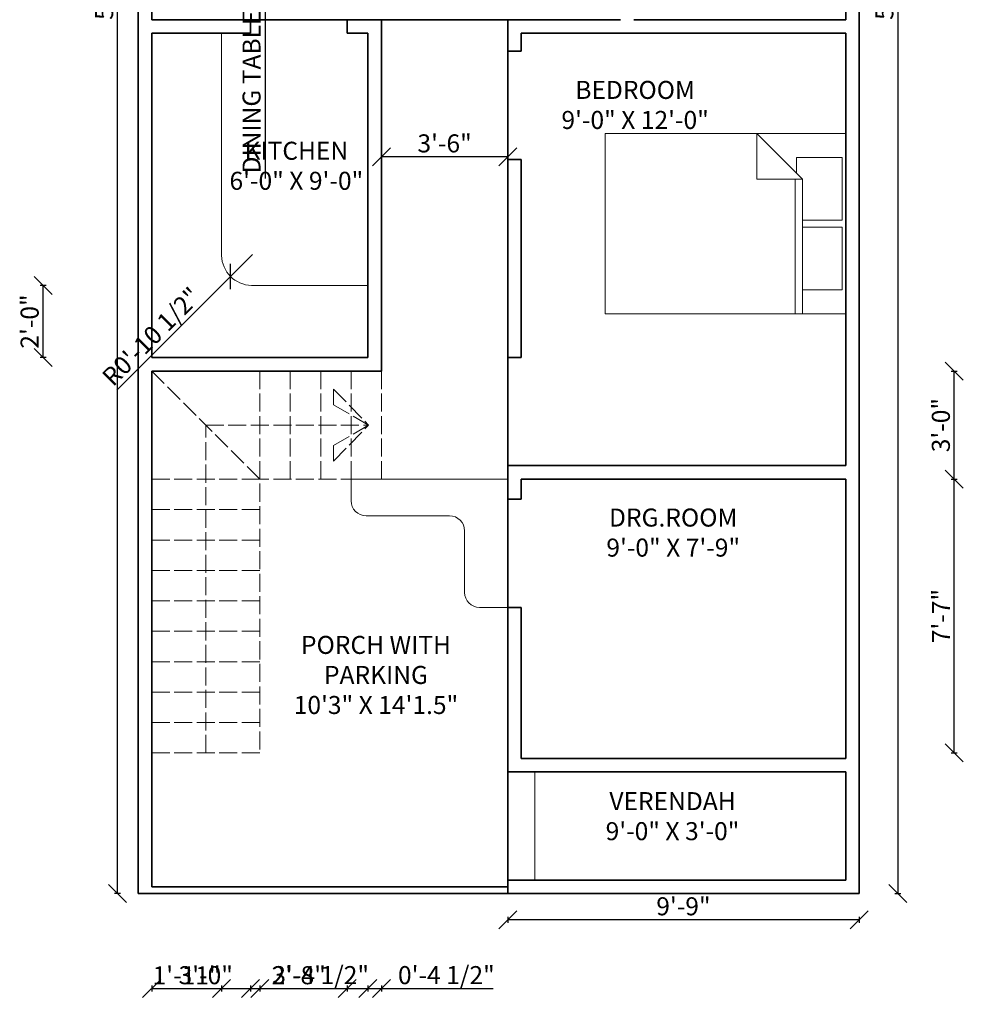
# Model space of a CAD drawing. Units: inches. Extents: x 2598 to 3019, y 330 to 985.
# Tile 1 of 2: x 2650 to 2964, y 330 to 657. Entities that reach past the tile are written whole.
import ezdxf

# ---------------------------------------------------------------- set-up
doc = ezdxf.new("R2010")
doc.units = ezdxf.units.IN
doc.linetypes.add('ACAD_ISO02W100', pattern=[15, 12, -3])
for name, color, linetype, lineweight in [('A-ANNO-DIMS', 2, 'Continuous', 13), ('A-AREA-IDEN', 114, 'Continuous', 18), ('A-FLOR', 7, 'Continuous', 18), ('A-FLOR-CASE', 8, 'Continuous', 18), ('A-FLOR-STRS', 212, 'ACAD_ISO02W100', 18), ('A-FURN', 8, 'Continuous', 18), ('A-WALL', 7, 'Continuous', 35)]:
    doc.layers.add(name, color=color, linetype=linetype, lineweight=lineweight)
doc.styles.get("Standard").update_dxf_attribs({"font": 'arial.ttf'})
doc.dimstyles.new('ISO-25', dxfattribs={"dimtxt": 6, "dimasz": 6, "dimexe": 1, "dimexo": 3, "dimtad": 1, "dimlunit": 3, "dimtxsty": 'Standard', "dimblk": 'OBLIQUE', "dimcen": 2.5, "dimclrt": 6, "dimadec": 0, "dimazin": 0, "dimtfac": 1, "dimtmove": 0, "dimatfit": 3, "dimfxl": 1, "dimfxlon": 1, "dimarcsym": 0})

# ---------------------------------------------------------------- blocks, each defined once
blk = doc.blocks.new('_Oblique')
at = {"color": 0, "linetype": 'ByBlock', "lineweight": -2}
blk.add_line((-0.5, -0.5), (0.5, 0.5), dxfattribs=at)
blk = doc.blocks.new('*D4')
at = {"layer": 'A-ANNO-DIMS', "color": 0, "lineweight": -2, "transparency": 16777216}
for p, q in [((2940.88, 970.94), (2942.88, 970.94)), ((2941.88, 970.94), (2941.88, 366.44)), ((2940.88, 366.44), (2942.88, 366.44))]:
    blk.add_line(p, q, dxfattribs=at)
at = {"layer": 'Defpoints', "color": 0, "transparency": 16777216}
for p in [(2929.06, 970.94), (2929.06, 366.44), (2941.88, 366.44)]:
    blk.add_point(p, dxfattribs=at)
at = {"layer": 'A-ANNO-DIMS', "color": 0, "lineweight": -2, "transparency": 16777216, "xscale": 6, "yscale": 6, "zscale": 6}
for p, rotation in [((2941.88, 970.94), 90), ((2941.88, 366.44), 270)]:
    blk.add_blockref('_Oblique', p, dxfattribs=dict(at, rotation=rotation))
at = {"layer": 'A-ANNO-DIMS', "color": 0, "transparency": 16777216, "insert": (2938.2, 668.69), "char_height": 6, "attachment_point": 5, "rotation": 90}
blk.add_mtext('50\'-0"', dxfattribs=at)
blk = doc.blocks.new('*D5')
at = {"layer": 'A-ANNO-DIMS', "color": 0, "lineweight": -2, "transparency": 16777216}
for p, q in [((2770.06, 611.78), (2770.06, 612.78)), ((2812.06, 611.78), (2770.06, 611.78)), ((2812.06, 611.78), (2812.06, 612.78))]:
    blk.add_line(p, q, dxfattribs=at)
at = {"layer": 'Defpoints', "color": 0, "transparency": 16777216}
for p in [(2770.06, 611.78), (2770.06, 610.94), (2812.06, 610.94)]:
    blk.add_point(p, dxfattribs=at)
at = {"layer": 'A-ANNO-DIMS', "color": 0, "lineweight": -2, "transparency": 16777216, "xscale": 6, "yscale": 6, "zscale": 6, "rotation": 180}
blk.add_blockref('_Oblique', (2770.06, 611.78), dxfattribs=at)
at = {"layer": 'A-ANNO-DIMS', "color": 0, "lineweight": -2, "transparency": 16777216, "xscale": 6, "yscale": 6, "zscale": 6}
blk.add_blockref('_Oblique', (2812.06, 611.78), dxfattribs=at)
at = {"layer": 'A-ANNO-DIMS', "color": 0, "transparency": 16777216, "insert": (2791.06, 615.48), "char_height": 6, "attachment_point": 5}
blk.add_mtext('3\'-6"', dxfattribs=at)
blk = doc.blocks.new('*D6')
at = {"layer": 'A-ANNO-DIMS', "color": 0, "lineweight": -2, "transparency": 16777216}
for p, q in [((2812.06, 358.75), (2812.06, 356.75)), ((2929.06, 357.75), (2812.06, 357.75)), ((2929.06, 358.75), (2929.06, 356.75))]:
    blk.add_line(p, q, dxfattribs=at)
at = {"layer": 'Defpoints', "color": 0, "transparency": 16777216}
for p in [(2812.06, 366.44), (2929.06, 366.44), (2812.06, 357.75)]:
    blk.add_point(p, dxfattribs=at)
at = {"layer": 'A-ANNO-DIMS', "color": 0, "lineweight": -2, "transparency": 16777216, "xscale": 6, "yscale": 6, "zscale": 6, "rotation": 180}
blk.add_blockref('_Oblique', (2812.06, 357.75), dxfattribs=at)
at = {"layer": 'A-ANNO-DIMS', "color": 0, "lineweight": -2, "transparency": 16777216, "xscale": 6, "yscale": 6, "zscale": 6}
blk.add_blockref('_Oblique', (2929.06, 357.75), dxfattribs=at)
at = {"layer": 'A-ANNO-DIMS', "color": 0, "transparency": 16777216, "insert": (2870.56, 361.44), "char_height": 6, "attachment_point": 5}
blk.add_mtext('9\'-9"', dxfattribs=at)
blk = doc.blocks.new('Bed - Queen')
for p, q in [((0, -80.00003), (0, 0)), ((0, 0), (59.99999, 0)), ((59.99999, 0), (59.99999, -80.00003)), ((7.99999, -1.2), (28.79998, -1.2)), ((7.99999, -14.4), (7.99999, -1.2)), ((28.79998, -1.2), (28.79998, -14.4)), ((31.19999, -1.2), (51.99999, -1.2)), ((31.19999, -14.4), (31.19999, -1.2)), ((51.99999, -1.2), (51.99999, -16.4)), ((0, -14.4), (44.8, -14.4)), ((59.99999, -29.6), (44.8, -14.4)), ((44.8, -14.4), (44.8, -29.6)), ((44.8, -16.8), (0, -16.8)), ((51.99999, -16.4), (46.79936, -16.4)), ((44.8, -29.6), (59.99999, -29.6)), ((59.99999, -80.00003), (0, -80.00003))]:
    blk.add_line(p, q)
blk = doc.blocks.new('*D15')
at = {"layer": 'A-ANNO-DIMS', "color": 0, "lineweight": -2, "transparency": 16777216}
for p, q in [((2683.19, 970.94), (2681.19, 970.94)), ((2682.19, 366.44), (2682.19, 970.94)), ((2683.19, 366.44), (2681.19, 366.44))]:
    blk.add_line(p, q, dxfattribs=at)
at = {"layer": 'Defpoints', "color": 0, "transparency": 16777216}
for p in [(2682.19, 970.94), (2689.06, 970.94), (2689.06, 366.44)]:
    blk.add_point(p, dxfattribs=at)
at = {"layer": 'A-ANNO-DIMS', "color": 0, "lineweight": -2, "transparency": 16777216, "xscale": 6, "yscale": 6, "zscale": 6}
for p, rotation in [((2682.19, 970.94), 90), ((2682.19, 366.44), 270)]:
    blk.add_blockref('_Oblique', p, dxfattribs=dict(at, rotation=rotation))
at = {"layer": 'A-ANNO-DIMS', "color": 0, "transparency": 16777216, "insert": (2678.5, 668.69), "char_height": 6, "attachment_point": 5, "rotation": 90}
blk.add_mtext('50\'-0"', dxfattribs=at)
blk = doc.blocks.new('*D25')
at = {"layer": 'A-ANNO-DIMS', "color": 0, "lineweight": -2, "transparency": 16777216}
for p, q in [((2732.31, 748.04), (2730.31, 748.04)), ((2731.31, 748.04), (2731.31, 688.04)), ((2732.31, 688.04), (2730.31, 688.04)), ((2731.31, 688.04), (2731.31, 604.59))]:
    blk.add_line(p, q, dxfattribs=at)
at = {"layer": 'Defpoints', "color": 0, "transparency": 16777216}
for p in [(2740.31, 748.04), (2731.31, 688.04), (2740.31, 688.04)]:
    blk.add_point(p, dxfattribs=at)
at = {"layer": 'A-ANNO-DIMS', "color": 0, "lineweight": -2, "transparency": 16777216, "xscale": 6, "yscale": 6, "zscale": 6}
for p, rotation in [((2731.31, 748.04), 90), ((2731.31, 688.04), 270)]:
    blk.add_blockref('_Oblique', p, dxfattribs=dict(at, rotation=rotation))
at = {"layer": 'A-ANNO-DIMS', "color": 6, "transparency": 16777216, "insert": (2727.58, 643.32), "char_height": 6, "attachment_point": 5, "rotation": 90}
blk.add_mtext('DINING TABLE 5\'-0"', dxfattribs=at)
blk = doc.blocks.new('*D27')
at = {"layer": 'A-ANNO-DIMS', "color": 0, "lineweight": -2, "transparency": 16777216}
for p, q in [((2693.56, 335.79), (2693.56, 333.79)), ((2693.56, 334.79), (2729.56, 334.79)), ((2729.56, 335.79), (2729.56, 333.79))]:
    blk.add_line(p, q, dxfattribs=at)
at = {"layer": 'Defpoints', "color": 0, "transparency": 16777216}
for p in [(2693.56, 413.27), (2729.56, 413.27), (2729.56, 334.79)]:
    blk.add_point(p, dxfattribs=at)
at = {"layer": 'A-ANNO-DIMS', "color": 0, "lineweight": -2, "transparency": 16777216, "xscale": 6, "yscale": 6, "zscale": 6, "rotation": 180}
blk.add_blockref('_Oblique', (2693.56, 334.79), dxfattribs=at)
at = {"layer": 'A-ANNO-DIMS', "color": 0, "lineweight": -2, "transparency": 16777216, "xscale": 6, "yscale": 6, "zscale": 6}
blk.add_blockref('_Oblique', (2729.56, 334.79), dxfattribs=at)
at = {"layer": 'A-ANNO-DIMS', "color": 6, "transparency": 16777216, "insert": (2711.56, 338.49), "char_height": 6, "attachment_point": 5}
blk.add_mtext('3\'-0"', dxfattribs=at)
blk = doc.blocks.new('*D28')
at = {"layer": 'A-ANNO-DIMS', "color": 0, "lineweight": -2, "transparency": 16777216}
for p, q in [((2959.711602, 504.44461), (2961.711602, 504.44461)), ((2960.711602, 413.27461), (2960.711602, 504.44461)), ((2959.711602, 413.27461), (2961.711602, 413.27461))]:
    blk.add_line(p, q, dxfattribs=at)
at = {"layer": 'Defpoints', "color": 0, "transparency": 16777216}
for p in [(2729.561602, 504.44461), (2960.711602, 504.44461), (2729.561602, 413.27461)]:
    blk.add_point(p, dxfattribs=at)
at = {"layer": 'A-ANNO-DIMS', "color": 0, "lineweight": -2, "transparency": 16777216, "xscale": 6, "yscale": 6, "zscale": 6}
for p, rotation in [((2960.711602, 504.44461), 90), ((2960.711602, 413.27461), 270)]:
    blk.add_blockref('_Oblique', p, dxfattribs=dict(at, rotation=rotation))
at = {"layer": 'A-ANNO-DIMS', "color": 6, "transparency": 16777216, "insert": (2957.086602, 458.85961), "char_height": 6, "attachment_point": 5, "rotation": 90}
blk.add_mtext('7\'-7"', dxfattribs=at)
blk = doc.blocks.new('*D29')
at = {"layer": 'A-ANNO-DIMS', "color": 0, "lineweight": -2, "transparency": 16777216}
for p, q in [((2959.71, 540.44), (2961.71, 540.44)), ((2960.71, 504.44), (2960.71, 540.44)), ((2959.71, 504.44), (2961.71, 504.44))]:
    blk.add_line(p, q, dxfattribs=at)
at = {"layer": 'Defpoints', "color": 0, "transparency": 16777216}
for p in [(2770.06, 540.44), (2960.71, 540.44), (2770.06, 504.44)]:
    blk.add_point(p, dxfattribs=at)
at = {"layer": 'A-ANNO-DIMS', "color": 0, "lineweight": -2, "transparency": 16777216, "xscale": 6, "yscale": 6, "zscale": 6}
for p, rotation in [((2960.71, 540.44), 90), ((2960.71, 504.44), 270)]:
    blk.add_blockref('_Oblique', p, dxfattribs=dict(at, rotation=rotation))
at = {"layer": 'A-ANNO-DIMS', "color": 6, "transparency": 16777216, "insert": (2957.02, 522.44), "char_height": 6, "attachment_point": 5, "rotation": 90}
blk.add_mtext('3\'-0"', dxfattribs=at)
blk = doc.blocks.new('*D30')
at = {"layer": 'A-ANNO-DIMS', "color": 0, "lineweight": -2, "transparency": 16777216}
for p, q in [((2729.56, 335.79), (2729.56, 333.79)), ((2729.56, 334.79), (2770.06, 334.79)), ((2770.06, 335.79), (2770.06, 333.79))]:
    blk.add_line(p, q, dxfattribs=at)
at = {"layer": 'Defpoints', "color": 0, "transparency": 16777216}
for p in [(2729.56, 504.44), (2770.06, 504.44), (2770.06, 334.79)]:
    blk.add_point(p, dxfattribs=at)
at = {"layer": 'A-ANNO-DIMS', "color": 0, "lineweight": -2, "transparency": 16777216, "xscale": 6, "yscale": 6, "zscale": 6, "rotation": 180}
blk.add_blockref('_Oblique', (2729.56, 334.79), dxfattribs=at)
at = {"layer": 'A-ANNO-DIMS', "color": 0, "lineweight": -2, "transparency": 16777216, "xscale": 6, "yscale": 6, "zscale": 6}
blk.add_blockref('_Oblique', (2770.06, 334.79), dxfattribs=at)
at = {"layer": 'A-ANNO-DIMS', "color": 6, "transparency": 16777216, "insert": (2749.81, 338.52), "char_height": 6, "attachment_point": 5}
blk.add_mtext('3\'-4 1/2"', dxfattribs=at)
blk = doc.blocks.new('*D31')
at = {"layer": 'A-ANNO-DIMS', "color": 0, "lineweight": -2, "transparency": 16777216}
for p, q in [((2693.56, 335.79), (2693.56, 333.79)), ((2693.56, 334.79), (2716.8, 334.79)), ((2716.8, 335.79), (2716.8, 333.79))]:
    blk.add_line(p, q, dxfattribs=at)
at = {"layer": 'Defpoints', "color": 0, "transparency": 16777216}
for p in [(2693.56, 652.94), (2716.8, 652.94), (2716.8, 334.79)]:
    blk.add_point(p, dxfattribs=at)
at = {"layer": 'A-ANNO-DIMS', "color": 0, "lineweight": -2, "transparency": 16777216, "xscale": 6, "yscale": 6, "zscale": 6, "rotation": 180}
blk.add_blockref('_Oblique', (2693.56, 334.79), dxfattribs=at)
at = {"layer": 'A-ANNO-DIMS', "color": 0, "lineweight": -2, "transparency": 16777216, "xscale": 6, "yscale": 6, "zscale": 6}
blk.add_blockref('_Oblique', (2716.8, 334.79), dxfattribs=at)
at = {"layer": 'A-ANNO-DIMS', "color": 6, "transparency": 16777216, "insert": (2705.18, 338.43), "char_height": 6, "attachment_point": 5}
blk.add_mtext('1\'-11"', dxfattribs=at)
blk = doc.blocks.new('*D32')
at = {"layer": 'A-ANNO-DIMS', "color": 0, "lineweight": -2, "transparency": 16777216}
for p, q in [((2658.41, 568.94), (2656.41, 568.94)), ((2657.41, 544.94), (2657.41, 568.94)), ((2658.41, 544.94), (2656.41, 544.94))]:
    blk.add_line(p, q, dxfattribs=at)
at = {"layer": 'Defpoints', "color": 0, "transparency": 16777216}
for p in [(2657.41, 568.94), (2765.56, 568.94), (2765.56, 544.94)]:
    blk.add_point(p, dxfattribs=at)
at = {"layer": 'A-ANNO-DIMS', "color": 0, "lineweight": -2, "transparency": 16777216, "xscale": 6, "yscale": 6, "zscale": 6}
for p, rotation in [((2657.41, 568.94), 90), ((2657.41, 544.94), 270)]:
    blk.add_blockref('_Oblique', p, dxfattribs=dict(at, rotation=rotation))
at = {"layer": 'A-ANNO-DIMS', "color": 6, "transparency": 16777216, "insert": (2653.72, 556.94), "char_height": 6, "attachment_point": 5, "rotation": 90}
blk.add_mtext('2\'-0"', dxfattribs=at)
blk = doc.blocks.new('*D33')
at = {"layer": 'A-ANNO-DIMS', "color": 0, "lineweight": -2, "transparency": 16777216}
for p, q in [((2726.42, 335.79), (2726.42, 333.79)), ((2726.42, 334.79), (2758.6, 334.79)), ((2758.6, 335.79), (2758.6, 333.79))]:
    blk.add_line(p, q, dxfattribs=at)
at = {"layer": 'Defpoints', "color": 0, "transparency": 16777216}
for p in [(2726.42, 652.94), (2758.6, 652.94), (2758.6, 334.79)]:
    blk.add_point(p, dxfattribs=at)
at = {"layer": 'A-ANNO-DIMS', "color": 0, "lineweight": -2, "transparency": 16777216, "xscale": 6, "yscale": 6, "zscale": 6, "rotation": 180}
blk.add_blockref('_Oblique', (2726.42, 334.79), dxfattribs=at)
at = {"layer": 'A-ANNO-DIMS', "color": 0, "lineweight": -2, "transparency": 16777216, "xscale": 6, "yscale": 6, "zscale": 6}
blk.add_blockref('_Oblique', (2758.6, 334.79), dxfattribs=at)
at = {"layer": 'A-ANNO-DIMS', "color": 6, "transparency": 16777216, "insert": (2742.51, 338.48), "char_height": 6, "attachment_point": 5}
blk.add_mtext('2\'-8"', dxfattribs=at)
blk = doc.blocks.new('*D34')
at = {"layer": 'A-ANNO-DIMS', "color": 0, "lineweight": -2, "transparency": 16777216}
for p, q in [((2765.56, 335.79), (2765.56, 333.79)), ((2765.56, 334.79), (2770.06, 334.79)), ((2770.06, 335.79), (2770.06, 333.79)), ((2770.06, 334.79), (2807.24, 334.79))]:
    blk.add_line(p, q, dxfattribs=at)
at = {"layer": 'Defpoints', "color": 0, "transparency": 16777216}
for p in [(2765.56, 544.94), (2770.06, 540.44), (2770.06, 334.79)]:
    blk.add_point(p, dxfattribs=at)
at = {"layer": 'A-ANNO-DIMS', "color": 0, "lineweight": -2, "transparency": 16777216, "xscale": 6, "yscale": 6, "zscale": 6, "rotation": 180}
blk.add_blockref('_Oblique', (2765.56, 334.79), dxfattribs=at)
at = {"layer": 'A-ANNO-DIMS', "color": 0, "lineweight": -2, "transparency": 16777216, "xscale": 6, "yscale": 6, "zscale": 6}
blk.add_blockref('_Oblique', (2770.06, 334.79), dxfattribs=at)
at = {"layer": 'A-ANNO-DIMS', "color": 6, "transparency": 16777216, "insert": (2791.65, 338.52), "char_height": 6, "attachment_point": 5}
blk.add_mtext('0\'-4 1/2"', dxfattribs=at)
blk = doc.blocks.new('*D39')
at = {"layer": 'A-ANNO-DIMS', "color": 0, "lineweight": -2, "transparency": 16777216}
for p in [(2727.08, 579.22), (2681.92, 534.06)]:
    blk.add_line(p, (2719.81, 571.95), dxfattribs=at)
at = {"layer": 'Defpoints', "color": 0, "transparency": 16777216}
for p in [(2727.08, 579.22), (2719.81, 571.95)]:
    blk.add_point(p, dxfattribs=at)
at = {"layer": 'A-ANNO-DIMS', "color": 0, "lineweight": -2, "transparency": 16777216, "xscale": 6, "yscale": 6, "zscale": 6, "rotation": 44.99835699208987}
blk.add_blockref('_Oblique', (2719.81, 571.95), dxfattribs=at)
at = {"layer": 'A-ANNO-DIMS', "color": 6, "transparency": 16777216, "insert": (2693.99, 551.4), "char_height": 6, "attachment_point": 5, "rotation": 44.9984}
blk.add_mtext('R0\'-10 1/2"', dxfattribs=at)

msp = doc.modelspace()

# ---------------------------------------------------------------- linework, layer by layer
at = {"layer": 'A-FLOR'}
for p, q in [((2759.937, 504.445), (2812.062, 504.445)), ((2759.937, 504.445), (2759.937, 497.246)), ((2764.937, 492.246), (2792.719, 492.246)), ((2797.719, 487.246), (2797.719, 466.758)), ((2802.719, 461.758), (2812.062, 461.758)), ((2821.062, 370.945), (2821.062, 406.945))]:
    msp.add_line(p, q, dxfattribs=at)
for centre, start, end in [((2764.937, 497.246), 180, 270), ((2792.719, 487.246), 0, 90), ((2802.719, 466.758), 180, 270)]:
    msp.add_arc(centre, 5, start, end, dxfattribs=at)
at = {"layer": 'A-FLOR-CASE'}
for p, q in [((2716.803, 652.945), (2716.803, 578.945)), ((2726.803, 568.945), (2765.562, 568.945))]:
    msp.add_line(p, q, dxfattribs=at)
msp.add_arc((2727.082, 579.223), 10.283, 181.55394, 268.44606, dxfattribs=at)
at = {"layer": 'A-FLOR-STRS', "ltscale": 0.5}
for p, q in [((2729.562, 504.445), (2693.562, 540.445)), ((2729.562, 540.445), (2729.562, 413.275)), ((2739.687, 540.445), (2739.687, 504.445)), ((2749.812, 540.445), (2749.812, 504.445)), ((2759.937, 540.445), (2759.937, 504.445)), ((2770.062, 540.445), (2770.062, 504.445)), ((2754.07, 534.446), (2765.776, 522.445)), ((2765.776, 522.445), (2754.07, 529.203)), ((2711.562, 413.275), (2711.562, 522.445)), ((2711.562, 522.445), (2765.776, 522.445)), ((2765.776, 522.445), (2754.07, 515.686)), ((2754.07, 510.443), (2765.776, 522.445)), ((2754.07, 515.686), (2754.07, 510.443)), ((2729.562, 504.445), (2693.562, 504.445)), ((2770.062, 504.445), (2729.562, 504.445)), ((2729.562, 494.315), (2693.562, 494.315)), ((2729.562, 484.185), (2693.562, 484.185)), ((2729.562, 474.055), (2693.562, 474.055)), ((2729.562, 463.925), (2693.562, 463.925)), ((2729.562, 453.795), (2693.562, 453.795)), ((2729.562, 443.665), (2693.562, 443.665)), ((2729.562, 433.535), (2693.562, 433.535)), ((2729.562, 423.405), (2693.562, 423.405)), ((2729.562, 413.275), (2693.562, 413.275))]:
    msp.add_line(p, q, dxfattribs=at)
at = {"layer": 'A-FLOR-STRS'}
msp.add_line((2754.07, 529.203), (2754.07, 534.446), dxfattribs=at)
at = {"layer": 'A-WALL'}
for p, q in [((2689.062, 970.945), (2689.062, 366.445)), ((2929.062, 366.445), (2929.062, 970.945)), ((2693.562, 777.445), (2693.562, 657.445)), ((2924.562, 657.445), (2924.562, 777.445)), ((2849.562, 657.445), (2693.562, 657.445)), ((2726.421, 652.945), (2726.421, 657.445)), ((2758.596, 652.945), (2758.596, 657.445)), ((2770.062, 657.445), (2770.062, 540.445)), ((2812.062, 504.445), (2812.062, 657.445)), ((2924.562, 657.445), (2854.062, 657.445)), ((2693.562, 652.945), (2693.562, 544.945)), ((2726.421, 652.945), (2693.562, 652.945)), ((2765.562, 652.945), (2758.596, 652.945)), ((2765.562, 652.945), (2765.562, 544.945)), ((2924.562, 652.945), (2816.562, 652.945)), ((2816.562, 646.945), (2816.562, 652.945)), ((2924.562, 508.945), (2924.562, 652.945)), ((2812.062, 646.945), (2816.562, 646.945)), ((2812.062, 610.945), (2816.562, 610.945)), ((2816.562, 544.945), (2816.562, 610.945)), ((2765.562, 544.945), (2693.562, 544.945)), ((2812.062, 544.945), (2816.562, 544.945)), ((2770.062, 540.445), (2693.562, 540.445)), ((2693.562, 540.445), (2693.562, 368.695)), ((2924.562, 508.945), (2812.062, 508.945)), ((2812.062, 406.945), (2812.062, 504.445)), ((2924.562, 504.445), (2816.562, 504.445)), ((2816.562, 497.758), (2816.562, 504.445)), ((2924.562, 411.445), (2924.562, 504.445)), ((2812.062, 497.758), (2816.562, 497.758)), ((2812.062, 461.758), (2816.562, 461.758)), ((2816.562, 411.445), (2816.562, 461.758)), ((2924.562, 411.445), (2816.562, 411.445)), ((2924.562, 406.945), (2812.062, 406.945)), ((2812.062, 366.445), (2812.062, 406.945)), ((2924.562, 370.945), (2924.562, 406.945)), ((2812.062, 370.945), (2924.562, 370.945)), ((2693.562, 368.695), (2812.062, 368.695)), ((2689.062, 366.445), (2929.062, 366.445))]:
    msp.add_line(p, q, dxfattribs=at)

# ---------------------------------------------------------------- block references
at = {"layer": 'A-FURN', "xscale": -1, "rotation": 270}
msp.add_blockref('Bed - Queen', (2924.562, 559.516), dxfattribs=at)

# ---------------------------------------------------------------- texts
at = {"layer": 'A-AREA-IDEN', "char_height": 6, "attachment_point": 1}
for s, insert in [('\\pxqc;BEDROOM\\P9\'-0" X 12\'-0"', (2821.296, 637.061)), ('\\pxqc;KITCHEN\\P6\'-0" X 9\'-0"', (2708.539, 616.799)), ('\\pxqc;DRG.ROOM\\P9\'-0" X 7\'-9"', (2833.979, 494.659)), ('\\pxqc;PORCH WITH\\PPARKING\\P10\'3" X 14\'1.5"', (2735.038, 452.249)), ('\\pxqc;VERENDAH\\P9\'-0" X 3\'-0"', (2833.74, 400.231))]:
    msp.add_mtext_dynamic_manual_height_columns(s, width=66.36505, gutter_width=12.5, heights=[0], dxfattribs=dict(at, insert=insert))

# ---------------------------------------------------------------- dimensions: what is measured, and where the dimension line sits
at = {"layer": 'A-ANNO-DIMS'}
for base, p1, p2, angle, text, override, picture, middle in [((2682.187, 970.945), (2689.062, 366.445), (2689.062, 970.945), 90, '50\'-0"', {"dimclrd": 0, "dimclre": 0, "dimclrt": 0}, '*D15', (2678.498, 668.695)), ((2941.884, 366.445), (2929.062, 970.945), (2929.062, 366.445), 90, '50\'-0"', {"dimclrd": 0, "dimclre": 0, "dimclrt": 0}, '*D4', (2938.195, 668.695)), ((2731.309, 688.042), (2740.309, 748.042), (2740.309, 688.042), 270, 'DINING TABLE <>', {"dimdec": 1, "dimlfac": 1, "dimrnd": 0, "dimzin": 1, "dimdsep": 46, "dimlunit": 4, "dimfrac": 2}, '*D25', (2727.582, 643.317))]:
    dim = msp.add_linear_dim(base=base, p1=p1, p2=p2, angle=angle, text=text, dimstyle='ISO-25', override=override, dxfattribs=at)
    dim.commit()
    dim.dimension.update_dxf_attribs({"geometry": picture, "text_midpoint": middle})
for base, p1, p2, override, picture, middle in [((2716.803, 334.795), (2693.562, 652.945), (2716.803, 652.945), {"dimdec": 1, "dimlfac": 1, "dimrnd": 0, "dimzin": 1, "dimdsep": 46, "dimlunit": 4, "dimfrac": 2}, '*D31', (2705.182, 338.432)), ((2758.596, 334.795), (2726.421, 652.945), (2758.596, 652.945), {"dimdec": 1, "dimlfac": 1, "dimrnd": 0, "dimzin": 1, "dimdsep": 46, "dimlunit": 4, "dimfrac": 2}, '*D33', (2742.509, 338.483)), ((2770.062, 611.785), (2812.062, 610.945), (2770.062, 610.945), {"dimclrd": 0, "dimclre": 0, "dimclrt": 0}, '*D5', (2791.062, 615.475)), ((2770.062, 334.795), (2765.562, 544.945), (2770.062, 540.445), {"dimdec": 1, "dimlfac": 1, "dimrnd": 0, "dimzin": 1, "dimdsep": 46, "dimlunit": 4, "dimfrac": 2}, '*D34', (2791.652, 338.522)), ((2770.062, 334.795), (2729.562, 504.445), (2770.062, 504.445), {"dimdec": 1, "dimlfac": 1, "dimrnd": 0, "dimzin": 1, "dimdsep": 46, "dimlunit": 4, "dimfrac": 2}, '*D30', (2749.812, 338.524)), ((2729.562, 334.795), (2693.562, 413.275), (2729.562, 413.275), {"dimdec": 1, "dimlfac": 1, "dimrnd": 0, "dimzin": 1, "dimdsep": 46, "dimlunit": 4, "dimfrac": 2}, '*D27', (2711.562, 338.485)), ((2812.062, 357.752), (2929.062, 366.445), (2812.062, 366.445), {"dimclrd": 0, "dimclre": 0, "dimclrt": 0}, '*D6', (2870.562, 361.44))]:
    dim = msp.add_linear_dim(base=base, p1=p1, p2=p2, dimstyle='ISO-25', override=override, dxfattribs=at)
    dim.commit()
    dim.dimension.update_dxf_attribs({"geometry": picture, "text_midpoint": middle})
dim = msp.add_radius_dim(center=(2727.082, 579.223), mpoint=(2719.811, 571.953), dimstyle='ISO-25', override={"dimdec": 1, "dimlfac": 1, "dimrnd": 0, "dimzin": 1, "dimdsep": 46, "dimlunit": 4, "dimfrac": 2}, dxfattribs=at)
dim.commit()
dim.dimension.update_dxf_attribs({"geometry": '*D39', "text_midpoint": (2693.987, 551.402)})
for base, p1, p2, picture, middle in [((2657.412, 568.945), (2765.562, 544.945), (2765.562, 568.945), '*D32', (2653.723, 556.945)), ((2960.712, 540.445), (2770.062, 504.445), (2770.062, 540.445), '*D29', (2957.021, 522.445)), ((2960.712, 504.445), (2729.562, 413.275), (2729.562, 504.445), '*D28', (2957.087, 458.86))]:
    dim = msp.add_linear_dim(base=base, p1=p1, p2=p2, angle=90, dimstyle='ISO-25', override={"dimdec": 1, "dimlfac": 1, "dimrnd": 0, "dimzin": 1, "dimdsep": 46, "dimlunit": 4, "dimfrac": 2}, dxfattribs=at)
    dim.commit()
    dim.dimension.update_dxf_attribs({"geometry": picture, "text_midpoint": middle})

doc.saveas('drawing.dxf')
